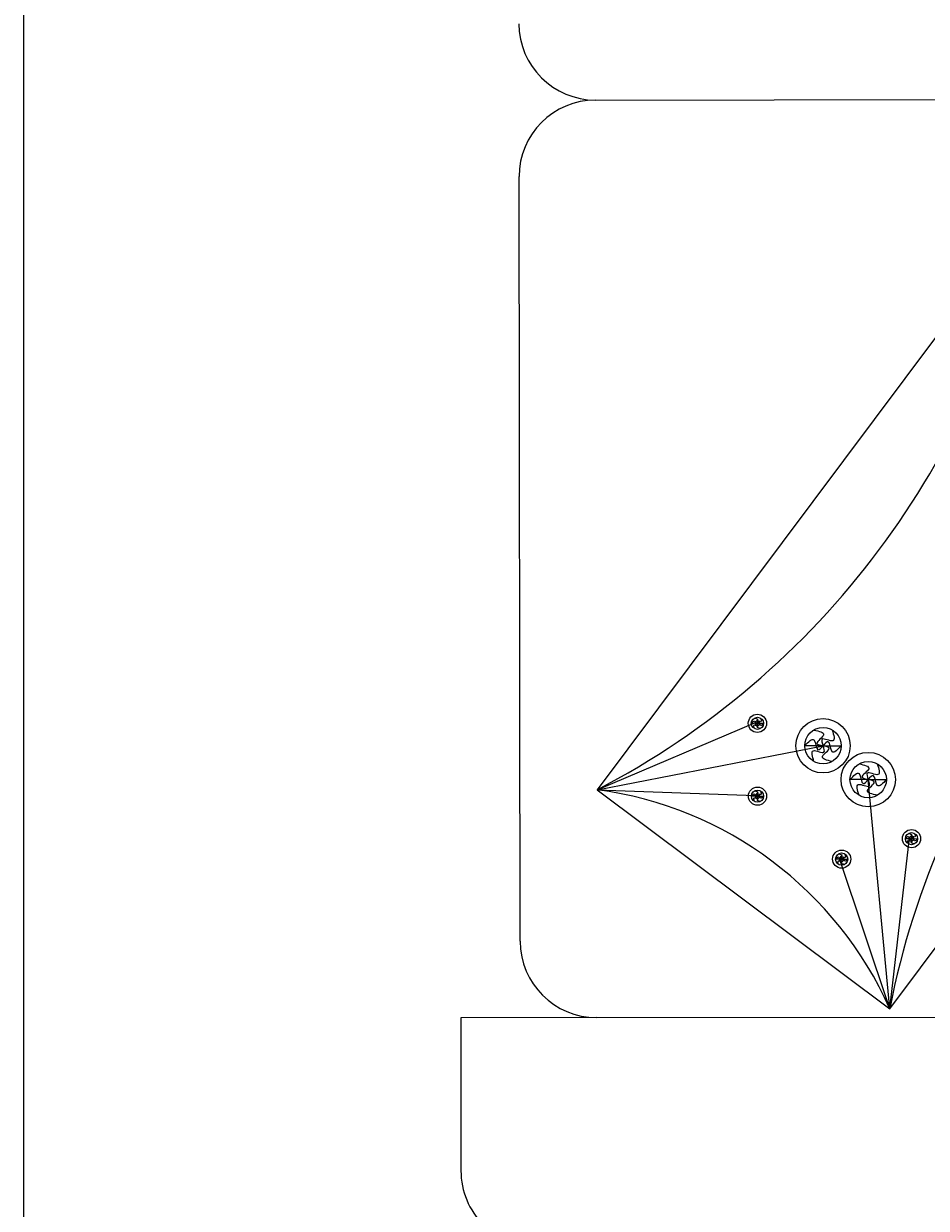
# Model space of a CAD drawing. Units: inches. Extents: x -61 to 1599, y -1316 to 257.
# Tile 136 of 204: x 492 to 515, y -135 to -104. Entities that reach past the tile are written whole.
import ezdxf

# ---------------------------------------------------------------- set-up
doc = ezdxf.new("R2010")
doc.units = ezdxf.units.IN
doc.header["$MEASUREMENT"] = 0
doc.layers.add('A-ANNO-DIMS', color=2, linetype='Continuous', lineweight=18)
doc.layers.add('FURNITURE', color=83, linetype='Continuous', lineweight=18)
doc.layers.add('FUR', color=83, linetype='Continuous')
doc.styles.get("Standard").update_dxf_attribs({"font": 'arial.ttf'})
doc.dimstyles.get("Standard").update_dxf_attribs({"dimtxt": 0.18, "dimasz": 0.18, "dimexe": 0.18, "dimexo": 0.0625, "dimgap": 0.09, "dimtad": 0, "dimtih": 1, "dimtoh": 1, "dimdec": 0, "dimzin": 0, "dimdsep": 46, "dimlunit": 3, "dimtxsty": 'Standard', "dimcen": 0.09, "dimadec": 0, "dimazin": 0, "dimtfac": 1, "dimtdec": 0, "dimtofl": 0, "dimtmove": 0, "dimatfit": 3, "dimfxl": 1, "dimtolj": 1, "dimtzin": 0, "dimarcsym": 0})

# ---------------------------------------------------------------- blocks, each defined once
blk = doc.blocks.new('*U227')
at = {"layer": 'FUR'}
blk.add_open_spline([(0.005, 0.08), (-0.03, 0.048), (-0.098, -0.015), (0.075, -0.018), (0.024, -0.063), (0.005, -0.08)], degree=3, knots=[0, 0, 0, 0, 0.0954578, 0.1898773, 0.2470677, 0.2470677, 0.2470677, 0.2470677], dxfattribs=at)
blk = doc.blocks.new('*U228')
at = {"layer": 'FURNITURE', "transparency": 16777216}
for p, rotation in [((222.173, -79.977), 60), ((222.312, -79.968), 300), ((222.178, -80.056), 120), ((222.25, -80.092), 180), ((222.317, -80.048), 240)]:
    blk.add_blockref('*U227', p, dxfattribs=dict(at, rotation=rotation))
blk.add_blockref('*U227', (222.24, -79.932), dxfattribs=at)
blk = doc.blocks.new('*U229')
at = {"layer": 'FUR'}
blk.add_open_spline([(0.005, 0.08), (-0.03, 0.048), (-0.098, -0.015), (0.075, -0.018), (0.024, -0.063), (0.005, -0.08)], degree=3, knots=[0, 0, 0, 0, 0.0954578, 0.1898773, 0.2470677, 0.2470677, 0.2470677, 0.2470677], dxfattribs=at)
blk = doc.blocks.new('*U230')
at = {"layer": 'FURNITURE', "transparency": 16777216}
for p, rotation in [((222.173, -79.977), 60), ((222.312, -79.968), 300), ((222.178, -80.056), 120), ((222.25, -80.092), 180), ((222.317, -80.048), 240)]:
    blk.add_blockref('*U229', p, dxfattribs=dict(at, rotation=rotation))
blk.add_blockref('*U229', (222.24, -79.932), dxfattribs=at)
blk = doc.blocks.new('*U231')
at = {"layer": 'FUR'}
blk.add_open_spline([(0.005, 0.08), (-0.03, 0.048), (-0.098, -0.015), (0.075, -0.018), (0.024, -0.063), (0.005, -0.08)], degree=3, knots=[0, 0, 0, 0, 0.0954578, 0.1898773, 0.2470677, 0.2470677, 0.2470677, 0.2470677], dxfattribs=at)
blk = doc.blocks.new('*U257')
at = {"layer": 'FURNITURE', "transparency": 16777216}
for p, rotation in [((222.173, -79.977), 60), ((222.312, -79.968), 300), ((222.178, -80.056), 120), ((222.25, -80.092), 180), ((222.317, -80.048), 240)]:
    blk.add_blockref('*U231', p, dxfattribs=dict(at, rotation=rotation))
blk.add_blockref('*U231', (222.24, -79.932), dxfattribs=at)
blk = doc.blocks.new('*U258')
at = {"layer": 'FUR'}
blk.add_open_spline([(0.005, 0.08), (-0.03, 0.048), (-0.098, -0.015), (0.075, -0.018), (0.024, -0.063), (0.005, -0.08)], degree=3, knots=[0, 0, 0, 0, 0.0954578, 0.1898773, 0.2470677, 0.2470677, 0.2470677, 0.2470677], dxfattribs=at)
blk = doc.blocks.new('*U259')
at = {"layer": 'FURNITURE', "transparency": 16777216}
for p, rotation in [((222.173, -79.977), 60), ((222.312, -79.968), 300), ((222.178, -80.056), 120), ((222.25, -80.092), 180), ((222.317, -80.048), 240)]:
    blk.add_blockref('*U258', p, dxfattribs=dict(at, rotation=rotation))
blk.add_blockref('*U258', (222.24, -79.932), dxfattribs=at)
blk = doc.blocks.new('*U260')
at = {"layer": 'FUR'}
blk.add_open_spline([(0.015, 0.238), (-0.088, 0.143), (-0.292, -0.045), (0.224, -0.053), (0.072, -0.187), (0.015, -0.238)], degree=3, knots=[0, 0, 0, 0, 0.2846533, 0.5662105, 0.736751, 0.736751, 0.736751, 0.736751], dxfattribs=at)
blk = doc.blocks.new('*U261')
at = {"layer": 'FURNITURE', "transparency": 16777216}
for p, rotation in [((662.517, -238.489), 60), ((662.929, -238.463), 300), ((662.531, -238.727), 120), ((662.944, -238.702), 240), ((662.745, -238.833), 180)]:
    blk.add_blockref('*U260', p, dxfattribs=dict(at, rotation=rotation))
blk.add_blockref('*U260', (662.716, -238.357), dxfattribs=at)
blk = doc.blocks.new('*U232')
at = {"layer": 'FUR'}
blk.add_open_spline([(0.015, 0.238), (-0.088, 0.143), (-0.292, -0.045), (0.224, -0.053), (0.072, -0.187), (0.015, -0.238)], degree=3, knots=[0, 0, 0, 0, 0.2846533, 0.5662105, 0.736751, 0.736751, 0.736751, 0.736751], dxfattribs=at)
blk = doc.blocks.new('*U256')
at = {"layer": 'FURNITURE', "transparency": 16777216}
for p, rotation in [((662.517, -238.489), 60), ((662.929, -238.463), 300), ((662.531, -238.727), 120), ((662.944, -238.702), 240), ((662.745, -238.833), 180)]:
    blk.add_blockref('*U232', p, dxfattribs=dict(at, rotation=rotation))
blk.add_blockref('*U232', (662.716, -238.357), dxfattribs=at)
blk = doc.blocks.new('*D704')
at = {"layer": 'A-ANNO-DIMS', "color": 0, "lineweight": -2, "transparency": 16777216}
for p, q in [((491.833, -616.882), (491.833, 257.457)), ((492.013, 257.277), (517.874, 257.277)), ((544.523, 257.277), (518.661, 257.277)), ((544.703, -616.882), (544.703, 257.457))]:
    blk.add_line(p, q, dxfattribs=at)
at = {"layer": 'A-ANNO-DIMS', "color": 0, "transparency": 16777216}
for points in [[(492.013, 257.307), (492.013, 257.247), (491.833, 257.277)], [(544.523, 257.307), (544.523, 257.247), (544.703, 257.277)]]:
    blk.add_solid(points, dxfattribs=at)
at = {"layer": 'DEFPOINTS', "color": 0, "transparency": 16777216}
for p in [(544.703, 257.277), (491.833, -616.945), (544.703, -616.945)]:
    blk.add_point(p, dxfattribs=at)
at = {"layer": 'A-ANNO-DIMS', "color": 0, "transparency": 16777216, "insert": (518.268, 257.277), "char_height": 0.18, "attachment_point": 5}
blk.add_mtext('\\A1;52.87', dxfattribs=at)

msp = doc.modelspace()

# ---------------------------------------------------------------- linework, layer by layer
at = {"layer": 'FURNITURE'}
for p, q in [((506.7909, -105.8149), (525.7629, -105.7888)), ((506.7909, -105.8149), (506.7909, -105.8149)), ((504.8212, -127.8176), (504.7937, -107.8176)), ((506.8361, -123.8538), (510.9754, -122.0981)), ((511.0279, -122.1174), (510.8681, -122.1176)), ((511.0279, -122.1174), (511.1877, -122.1172)), ((506.8361, -123.8538), (512.7451, -122.7042)), ((512.7451, -122.7042), (512.2686, -122.7048)), ((512.7451, -122.7042), (513.2216, -122.7035)), ((513.9261, -123.588), (513.4496, -123.5886)), ((513.9261, -123.588), (514.4026, -123.5873)), ((514.49, -129.5812), (513.9261, -123.588)), ((506.8361, -123.8538), (510.978, -124.0022)), ((511.0305, -124.0215), (510.8708, -124.0217)), ((511.0305, -124.0215), (511.1903, -124.0213)), ((514.49, -129.5812), (515.0068, -125.1148)), ((515.0593, -125.1341), (514.8995, -125.1343)), ((515.0593, -125.1341), (515.2191, -125.1338)), ((513.2318, -125.6687), (513.072, -125.6689)), ((514.49, -129.5812), (513.1793, -125.6494)), ((513.2318, -125.6687), (513.3915, -125.6685)), ((506.8239, -129.8148), (503.2659, -129.8197)), ((506.8239, -129.8148), (523.7958, -129.7915))]:
    msp.add_line(p, q, dxfattribs=at)
msp.add_lwpolyline([(503.2659, -129.8197), (503.2714, -133.8197, 0.4142136), (505.2742, -135.817), (527.2741, -135.7867, 0.4142137), (529.2714, -133.784), (529.1944, -77.784, 0.4142134), (527.1916, -75.7868), (505.1917, -75.817, 0.4142136), (503.1944, -77.8197), (503.1999, -81.8197)], format="xyb", dxfattribs=at)
msp.add_lwpolyline([(518.121, -108.7733), (506.8361, -123.8538), (514.49, -129.5812), (525.7748, -114.5007)], close=True, dxfattribs=at)
for centre, radius in [((511.0279, -122.1174), 0.2382), ((511.0279, -122.1174), 0.1598), ((512.7451, -122.7042), 0.7104), ((512.7451, -122.7042), 0.4765), ((513.9261, -123.588), 0.7104), ((513.9261, -123.588), 0.4765), ((511.0305, -124.0215), 0.2382), ((511.0305, -124.0215), 0.1598), ((515.0593, -125.1341), 0.2382), ((515.0593, -125.1341), 0.1598), ((513.2318, -125.6687), 0.2382), ((513.2318, -125.6687), 0.1598)]:
    msp.add_circle(centre, radius, dxfattribs=at)
for centre, radius, start, end in [((506.7882, -103.8149), 2, 180.07876, 270.07876), ((506.7937, -107.8149), 2, 90.07876, 180.07876), ((496.7984, -104.58), 21.731, 297.51039, 348.87432), ((535.8126, -133.7745), 21.731, 117.51039, 168.87432), ((505.5263, -133.5821), 9.816, 24.05298, 82.33173), ((506.8212, -127.8148), 2, 180.07876, 270.07876)]:
    msp.add_arc(centre, radius, start, end, dxfattribs=at)

# ---------------------------------------------------------------- block references
at = {"layer": 'FURNITURE', "xscale": -1, "rotation": 270.0787636990076}
for name, p in [('*U230', (591.3457, -344.2521)), ('*U261', (752.2511, -785.1057)), ('*U256', (753.4321, -785.9895)), ('*U228', (591.3483, -346.1563)), ('*U259', (595.3771, -347.2688)), ('*U257', (593.5495, -347.8034))]:
    msp.add_blockref(name, p, dxfattribs=at)

# ---------------------------------------------------------------- dimensions: what is measured, and where the dimension line sits
at = {"layer": 'A-ANNO-DIMS'}
dim = msp.add_linear_dim(base=(544.7028, 257.2771), p1=(491.8327, -616.9446), p2=(544.7028, -616.9446), dimstyle='Standard', override={"dimdec": 2, "dimlfac": 1, "dimrnd": 0, "dimzin": 0, "dimdsep": 46, "dimlunit": 2}, dxfattribs=at)
dim.commit()
dim.dimension.update_dxf_attribs({"geometry": '*D704', "text_midpoint": (518.2677, 257.2771)})

doc.saveas('drawing.dxf')
